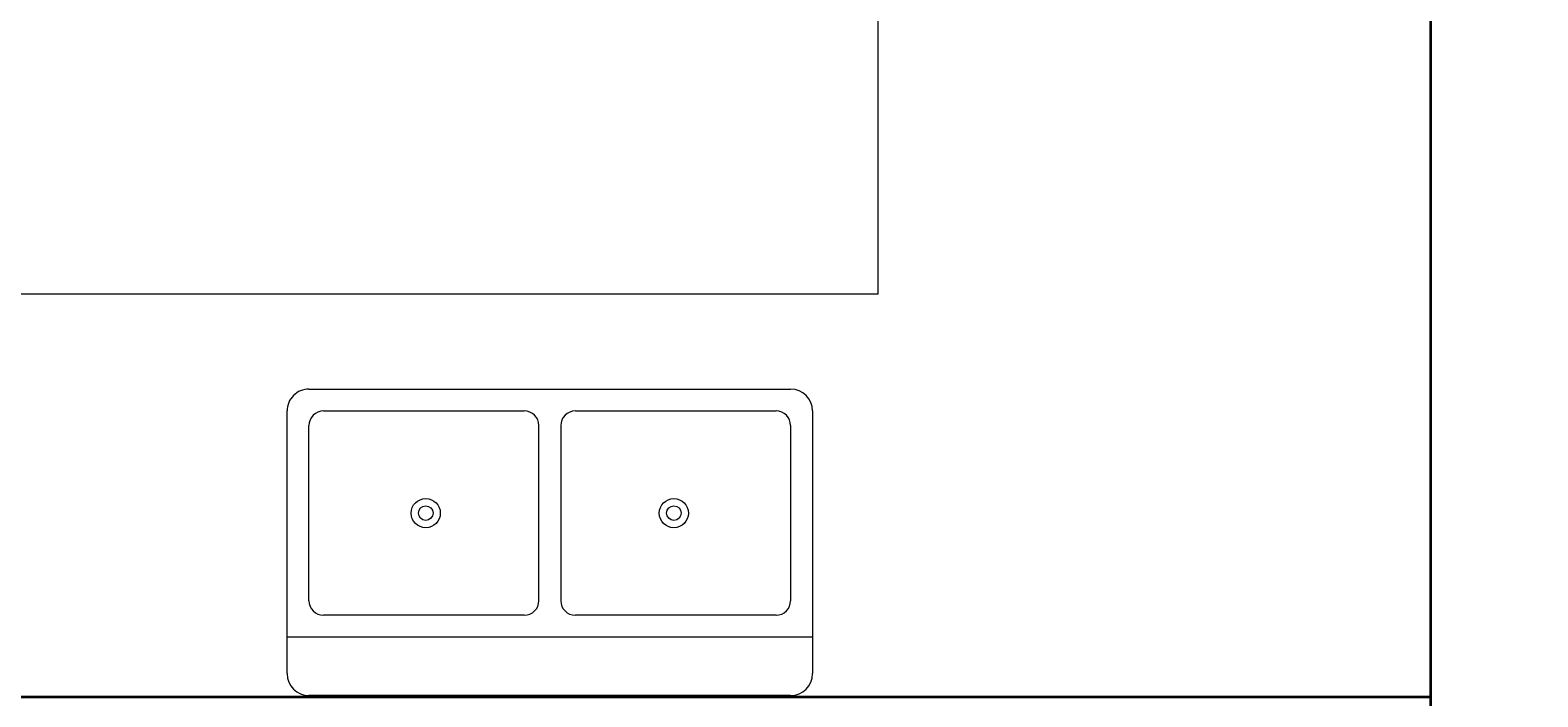
# Model space of a CAD drawing. Units: millimetres. Extents: x 27017497 to 27018854, y 7058029 to 7059154.
# Tile 50 of 91: x 27017962 to 27018038, y 7058203 to 7058236. Entities that reach past the tile are written whole.
import ezdxf

# ---------------------------------------------------------------- set-up
doc = ezdxf.new("R2010")
doc.units = ezdxf.units.MM
for name, color, linetype, lineweight in [('A-ANNO-DIMS', 2, 'Continuous', 18), ('A-FLOR-CASE', 8, 'Continuous', 20), ('A-FLOR-FIXT', 9, 'Continuous', 18), ('A-WALL', 7, 'Continuous', 35)]:
    doc.layers.add(name, color=color, linetype=linetype, lineweight=lineweight)
doc.styles.get("Standard").update_dxf_attribs({"font": 'arial.ttf'})
doc.dimstyles.get("Standard").update_dxf_attribs({"dimtxt": 0.18, "dimasz": 0.18, "dimexe": 0.18, "dimexo": 0.0625, "dimgap": 0.09, "dimtad": 0, "dimtih": 1, "dimtoh": 1, "dimdec": 4, "dimzin": 0, "dimdsep": 46, "dimtxsty": 'Standard', "dimcen": 0.09, "dimadec": 0, "dimazin": 0, "dimtfac": 1, "dimtdec": 4, "dimtofl": 0, "dimtmove": 0, "dimatfit": 3, "dimfxl": 1, "dimtolj": 1, "dimtzin": 0, "dimarcsym": 0})

# ---------------------------------------------------------------- blocks, each defined once
blk = doc.blocks.new('Sink-double - 36 in top')
for p, q in [((-18, -4), (18, -4)), ((-0.75, -18.5), (-0.75, -6.5)), ((0.75, -6.5), (0.75, -18.5))]:
    blk.add_line(p, q)
for points in [[(-16.5, 0), (16.5, 0)], [(-18, -19.5), (-18, -1.5)], [(18, -1.5), (18, -19.5)], [(-15.5, -5.5), (-1.75, -5.5)], [(1.75, -5.5), (15.5, -5.5)], [(-16.5, -18.5), (-16.5, -6.5)], [(16.5, -6.5), (16.5, -18.5)], [(-1.75, -19.5), (-15.5, -19.5)], [(15.5, -19.5), (1.75, -19.5)], [(16.5, -21), (-16.5, -21)]]:
    blk.add_lwpolyline(points)
for centre, radius in [((-8.5, -12.5), 1), ((-8.5, -12.5), 0.5), ((8.5, -12.5), 1), ((8.5, -12.5), 0.5)]:
    blk.add_circle(centre, radius)
for centre, radius, start, end in [((-16.5, -1.5), 1.5, 90, 180), ((16.5, -1.5), 1.5, 0, 90), ((-15.5, -6.5), 1, 90, 180), ((-1.75, -6.5), 1, 0, 90), ((1.75, -6.5), 1, 90, 180), ((15.5, -6.5), 1, 0, 90), ((-15.5, -18.5), 1, 180, 270), ((-1.75, -18.5), 1, 270, 0), ((1.75, -18.5), 1, 180, 270), ((15.5, -18.5), 1, 270, 0), ((-16.5, -19.5), 1.5, 180, 270), ((16.5, -19.5), 1.5, 270, 0)]:
    blk.add_arc(centre, radius, start, end)
blk = doc.blocks.new('*D47')
at = {"layer": 'A-ANNO-DIMS', "color": 0, "lineweight": -2, "transparency": 16777216}
for p, q in [((27017561.166, 7058294.35), (27017561.166, 7058028.6)), ((27018790.606, 7058294.35), (27018790.606, 7058028.6)), ((27017561.346, 7058028.78), (27018175.431, 7058028.78)), ((27018790.426, 7058028.78), (27018176.341, 7058028.78))]:
    blk.add_line(p, q, dxfattribs=at)
at = {"layer": 'A-ANNO-DIMS', "color": 0, "transparency": 16777216}
for points in [[(27017561.346, 7058028.81), (27017561.346, 7058028.75), (27017561.166, 7058028.78)], [(27018790.426, 7058028.81), (27018790.426, 7058028.75), (27018790.606, 7058028.78)]]:
    blk.add_solid(points, dxfattribs=at)
at = {"layer": 'Defpoints', "color": 0, "transparency": 16777216}
for p in [(27017561.166, 7058294.412), (27018790.606, 7058294.412), (27018790.606, 7058028.78)]:
    blk.add_point(p, dxfattribs=at)
at = {"layer": 'A-ANNO-DIMS', "color": 0, "transparency": 16777216, "insert": (27018175.886, 7058028.78), "char_height": 0.18, "attachment_point": 5}
blk.add_mtext('\\A1;1229.4', dxfattribs=at)
blk = doc.blocks.new('*D48')
at = {"layer": 'A-ANNO-DIMS', "color": 0, "lineweight": -2, "transparency": 16777216}
for p, q in [((27018463.498, 7058622.912), (27017497.536, 7058622.912)), ((27017497.716, 7058622.732), (27017497.716, 7058357.753)), ((27017497.716, 7058092.41), (27017497.716, 7058357.389)), ((27018555.129, 7058092.23), (27017497.536, 7058092.23))]:
    blk.add_line(p, q, dxfattribs=at)
at = {"layer": 'A-ANNO-DIMS', "color": 0, "transparency": 16777216}
for points in [[(27017497.686, 7058622.732), (27017497.746, 7058622.732), (27017497.716, 7058622.912)], [(27017497.686, 7058092.41), (27017497.746, 7058092.41), (27017497.716, 7058092.23)]]:
    blk.add_solid(points, dxfattribs=at)
at = {"layer": 'Defpoints', "color": 0, "transparency": 16777216}
for p in [(27018463.561, 7058622.912), (27017497.716, 7058092.23), (27018555.192, 7058092.23)]:
    blk.add_point(p, dxfattribs=at)
at = {"layer": 'A-ANNO-DIMS', "color": 0, "transparency": 16777216, "insert": (27017497.716, 7058357.571), "char_height": 0.18, "attachment_point": 5}
blk.add_mtext('\\A1;530.7', dxfattribs=at)

msp = doc.modelspace()

# ---------------------------------------------------------------- linework, layer by layer
at = {"layer": 'A-FLOR-CASE'}
for p, q in [((27018004.365, 7058294.322), (27018004.365, 7058223.172)), ((27018004.365, 7058223.172), (27017956.932, 7058223.172))]:
    msp.add_line(p, q, dxfattribs=at)
at = {"layer": 'A-WALL'}
for p, q in [((27018032.166, 7058386.803), (27018032.166, 7058141.912)), ((27017934.651, 7058202.912), (27018032.166, 7058202.912))]:
    msp.add_line(p, q, dxfattribs=at)

# ---------------------------------------------------------------- block references
at = {"layer": 'A-FLOR-FIXT', "xscale": 0.7340308267416257, "yscale": 0.7340308267416257, "zscale": 0.7340308267416257, "rotation": 180}
msp.add_blockref('Sink-double - 36 in top', (27017987.873, 7058202.978), dxfattribs=at)

# ---------------------------------------------------------------- dimensions: what is measured, and where the dimension line sits
at = {"layer": 'A-ANNO-DIMS'}
dim = msp.add_linear_dim(base=(27017497.716, 7058092.23), p1=(27018463.561, 7058622.912), p2=(27018555.192, 7058092.23), angle=90, dimstyle='Standard', override={"dimdec": 1, "dimlfac": 1, "dimrnd": 0, "dimzin": 0, "dimdsep": 46, "dimlunit": 2}, dxfattribs=at)
dim.commit()
dim.dimension.update_dxf_attribs({"geometry": '*D48', "text_midpoint": (27017497.716, 7058357.571)})
dim = msp.add_linear_dim(base=(27018790.606, 7058028.78), p1=(27017561.166, 7058294.412), p2=(27018790.606, 7058294.412), dimstyle='Standard', override={"dimdec": 1, "dimlfac": 1, "dimrnd": 0, "dimzin": 0, "dimdsep": 46, "dimlunit": 2}, dxfattribs=at)
dim.commit()
dim.dimension.update_dxf_attribs({"geometry": '*D47', "text_midpoint": (27018175.886, 7058028.78)})

doc.saveas('drawing.dxf')
